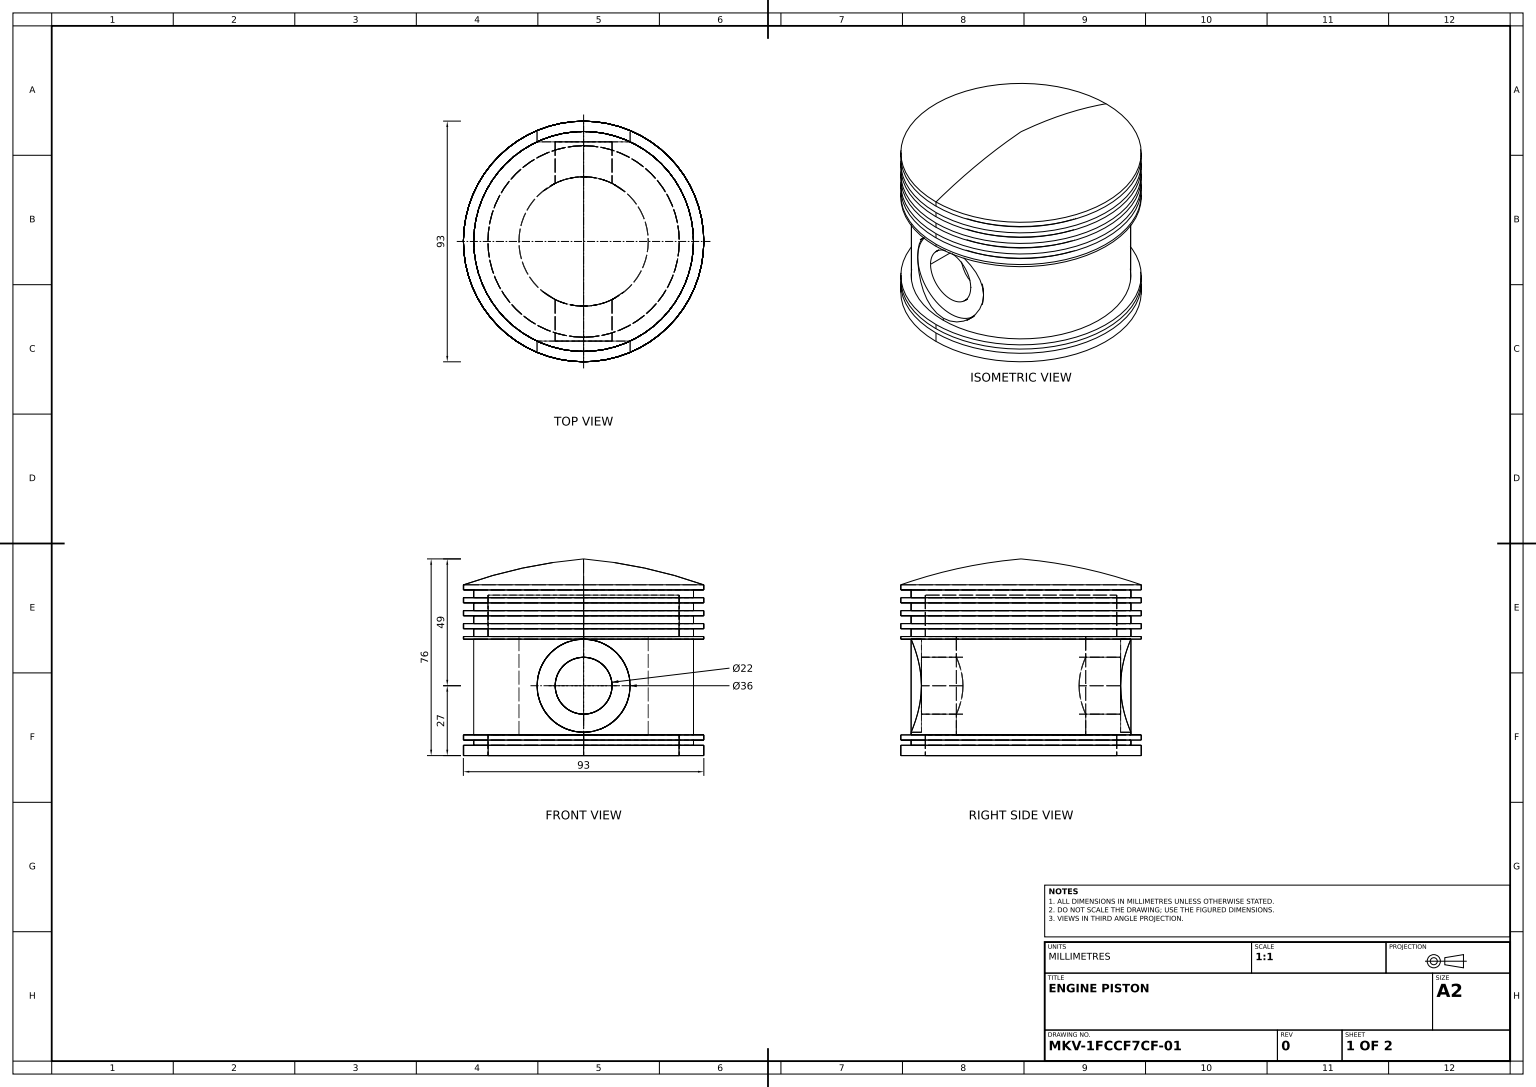
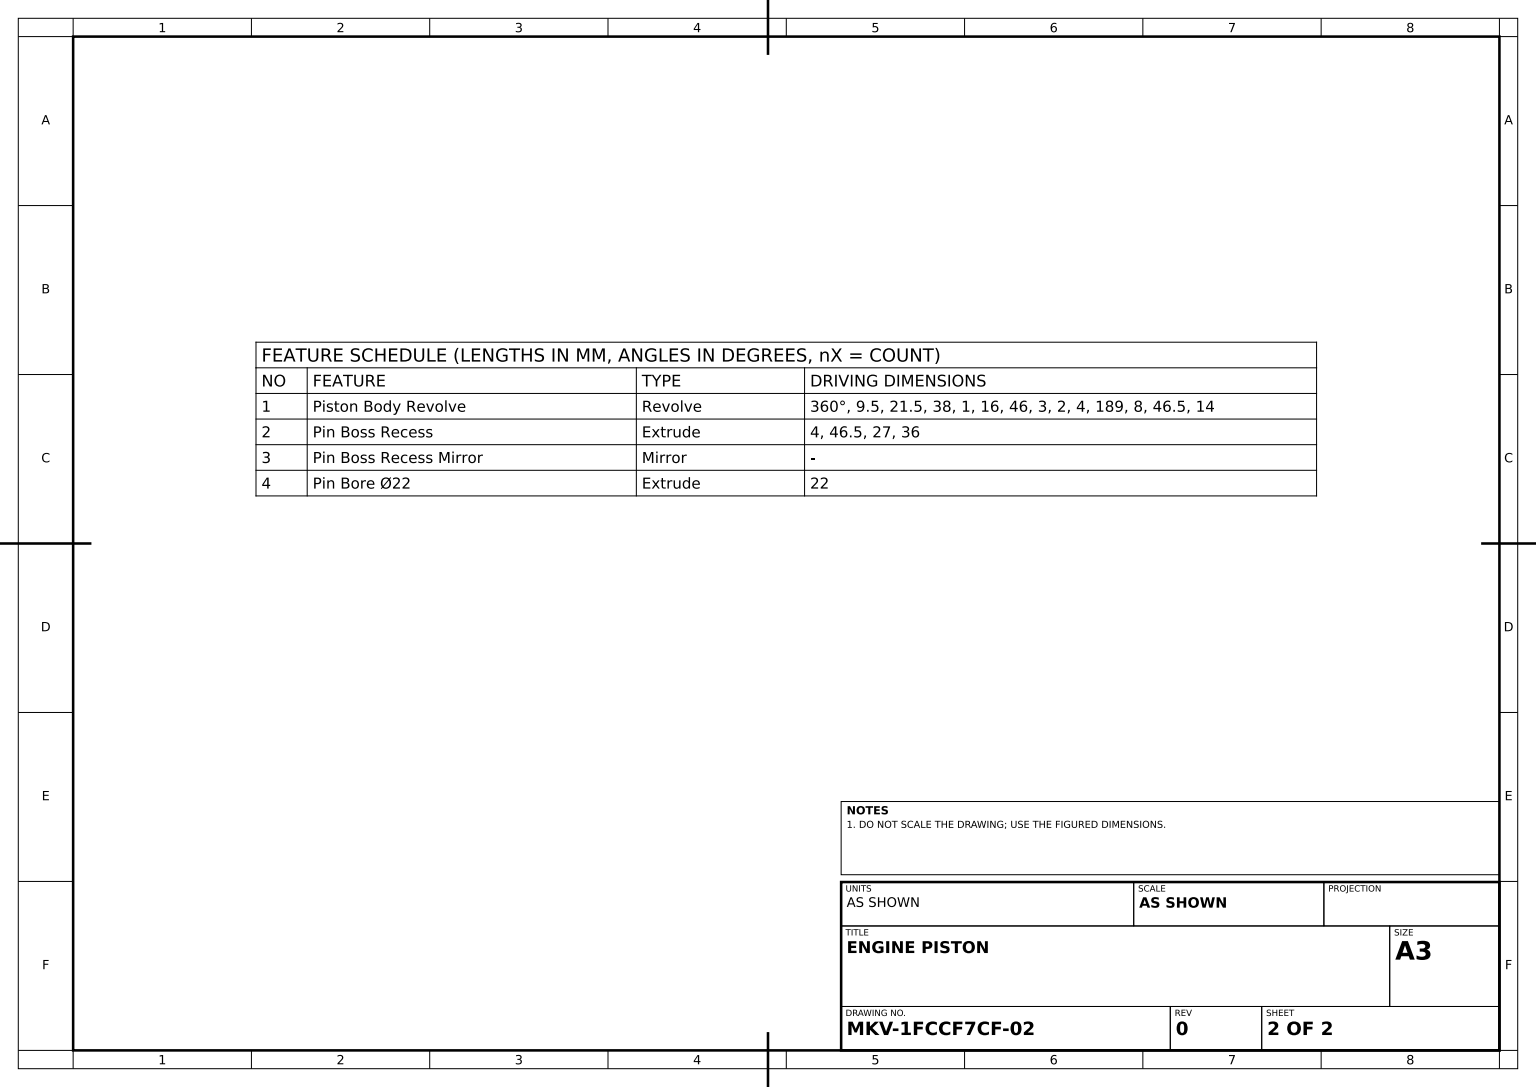
from build123d import *

# Parameters (mm, degrees)
PIN_BOSS_RECESS_SKETCH_R = 18
PIN_BOSS_RECESS_DEPTH    = 4
PIN_BORE_SKETCH_R        = 11
PIN_BORE_22_DEPTH        = 150.48578545


with BuildPart() as part:
    # Piston Profile Sketch → Piston Body Revolve (revolve)
    with BuildSketch(Plane.XY, mode=Mode.PRIVATE) as piston_body_revolve_sk:
        with BuildLine():
            Line((0, 0), (9.5, 0))
            Line((9.5, 0), (9.5, 8))
            Line((9.5, 8), (21.5, 8))
            Line((21.5, 8), (21.5, 46))
            Line((21.5, 46), (9.5, 46))
            Line((9.5, 46), (9.5, 62))
            Line((9.5, 62), (46.5, 62))
            Line((46.5, 62), (46.5, 76))
            ThreePointArc((46.5, 76), (22.934174039, 72.468590717), (0, 66))
            Line((0, 66), (0, 64))
            Line((0, 64), (4, 64))
            Line((4, 64), (4, 61))
            Line((4, 61), (0, 61))
            Line((0, 61), (0, 59))
            Line((0, 59), (4, 59))
            Line((4, 59), (4, 56))
            Line((4, 56), (0, 56))
            Line((0, 56), (0, 54))
            Line((0, 54), (4, 54))
            Line((4, 54), (4, 51))
            Line((4, 51), (0, 51))
            Line((0, 51), (0, 49))
            Line((0, 49), (4, 49))
            Line((4, 49), (4, 46))
            Line((4, 46), (0, 46))
            Line((0, 46), (0, 45))
            Line((0, 45), (4, 45))
            Line((4, 45), (4, 8))
            Line((4, 8), (0, 8))
            Line((0, 8), (0, 6))
            Line((0, 6), (4, 6))
            Line((4, 6), (4, 4))
            Line((4, 4), (0, 4))
            Line((0, 4), (0, 0))
        make_face()
    revolve(piston_body_revolve_sk.sketch.rotate(Axis((46.5, 0, 0), (0, 1, 0)), 270), axis=Axis((46.5, 0, 0), (0, 1, 0)))

    # Pin Boss Recess Sketch → Pin Boss Recess (cut)
    with BuildSketch(Plane.XY.offset(42.5)):
        with Locations((46.5, 27)):
            Circle(PIN_BOSS_RECESS_SKETCH_R)
    pin_boss_recess = extrude(amount=-PIN_BOSS_RECESS_DEPTH, mode=Mode.SUBTRACT)

    # Pin Boss Recess Mirror: Pin Boss Recess across plane
    add(pin_boss_recess.mirror(Plane.XY), mode=Mode.SUBTRACT)

    # Pin Bore Sketch → Pin Bore Ø22 (cut, through all)
    with BuildSketch(Plane.XY.offset(42.5)):
        with Locations(Location((46.5, 27, 0), (0, 0, 90))):
            Circle(PIN_BORE_SKETCH_R)
    extrude(amount=-PIN_BORE_22_DEPTH, mode=Mode.SUBTRACT)


solid = part.part
